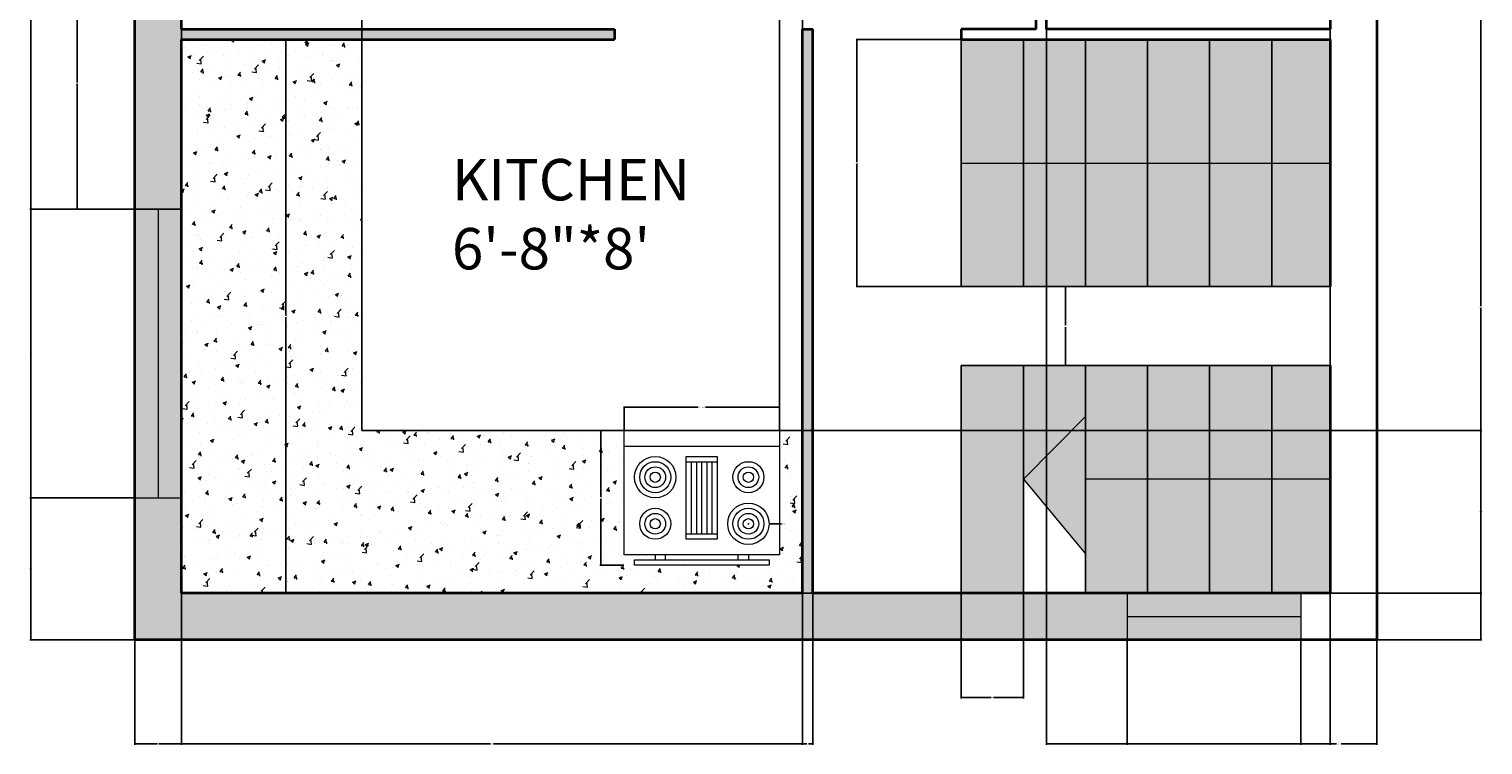
# Model space of a CAD drawing. Units: inches. Extents: x 17031430 to 17032061, y 16082759 to 16083238.
# Tile 1 of 3: x 17031435 to 17031716, y 16082759 to 16082898. Entities that reach past the tile are written whole.
import ezdxf

# ---------------------------------------------------------------- set-up
doc = ezdxf.new("R2010")
doc.units = ezdxf.units.IN
doc.header["$MEASUREMENT"] = 0
for name, color, linetype, lineweight in [('A-ANNO-DIMS', 2, 'Continuous', 18), ('A-AREA-IDEN', 7, 'Continuous', 25), ('A-EQPM', 8, 'Continuous', 18), ('A-FLOR-CASE', 8, 'Continuous', 25), ('A-FLOR-STRS', 7, 'Continuous', 25), ('A-FLOR-STRS-PATT', 254, 'Continuous', 13), ('A-GLAZ', 4, 'Continuous', 18), ('A-WALL', 7, 'Continuous', 35)]:
    doc.layers.add(name, color=color, linetype=linetype, lineweight=lineweight)
for name, color, linetype, lineweight, true_color in [('A-ANNO-SYMB', 116, 'Continuous', 18, 0x136734), ('A-ANNO-SYMB-PATT', 116, 'Continuous', 13, 0x136734), ('A-FLOR-CASE-PATT', 9, 'Continuous', 13, 0xc7c8ca), ('A-GLAZ-PATT', 252, 'Continuous', 13, 0x939598), ('A-WALL-PATT', 18, 'Continuous', 13, 0x000000)]:
    doc.layers.add(name, color=color, linetype=linetype, lineweight=lineweight, true_color=true_color)
doc.styles.get("Standard").update_dxf_attribs({"font": 'arial.ttf'})
doc.dimstyles.get("Standard").update_dxf_attribs({"dimtxt": 0.18, "dimasz": 0.18, "dimexe": 0.18, "dimexo": 0.0625, "dimgap": 0.09, "dimtad": 0, "dimtih": 1, "dimtoh": 1, "dimdec": 0, "dimzin": 0, "dimdsep": 46, "dimlunit": 3, "dimtxsty": 'Standard', "dimcen": 0.09, "dimadec": 0, "dimazin": 0, "dimtfac": 1, "dimtdec": 0, "dimtofl": 0, "dimtmove": 0, "dimatfit": 3, "dimfxl": 1, "dimtolj": 1, "dimtzin": 0, "dimarcsym": 0})

# ---------------------------------------------------------------- blocks, each defined once
blk = doc.blocks.new('Range-Oven - 30 in top')
for p, q in [((0, -3), (30, -3)), ((12, -6), (18, -6)), ((13, -20), (13, -6)), ((14, -6), (14, -20)), ((15, -20), (15, -6)), ((16, -6), (16, -20)), ((17, -20), (17, -6)), ((18, -20), (12, -20)), ((6, -24), (6, -25)), ((8, -25), (8, -24)), ((22, -25), (22, -24)), ((24, -24), (24, -25))]:
    blk.add_line(p, q)
for points in [[(0, -24), (0, 0), (30, 0), (30, -24)], [(12, -21), (12, -5), (18, -5), (18, -21)], [(2, -26), (2, -25), (28, -25), (28, -26)]]:
    blk.add_lwpolyline(points, close=True)
for centre, radius in [((6, -9), 4), ((6, -9), 3), ((6, -9), 2), ((6, -9), 1), ((24, -9), 3), ((24, -9), 2), ((24, -9), 1), ((24, -18), 4), ((6, -18), 3), ((6, -18), 2), ((24, -18), 3), ((24, -18), 2), ((6, -18), 1), ((24, -18), 1)]:
    blk.add_circle(centre, radius)
blk = doc.blocks.new('*D12')
at = {"layer": 'A-ANNO-DIMS', "color": 0, "lineweight": -2, "transparency": 16777216}
for p, q in [((17031550.32, 16082820.21), (17031550.32, 16082824.83)), ((17031550.5, 16082824.65), (17031564.62, 16082824.65)), ((17031580.14, 16082824.65), (17031566.01, 16082824.65)), ((17031580.32, 16082820.21), (17031580.32, 16082824.83))]:
    blk.add_line(p, q, dxfattribs=at)
at = {"layer": 'A-ANNO-DIMS', "color": 0, "transparency": 16777216}
for points in [[(17031550.5, 16082824.68), (17031550.5, 16082824.62), (17031550.32, 16082824.65)], [(17031580.14, 16082824.68), (17031580.14, 16082824.62), (17031580.32, 16082824.65)]]:
    blk.add_solid(points, dxfattribs=at)
at = {"layer": 'Defpoints', "color": 0, "transparency": 16777216}
for p in [(17031580.32, 16082824.65), (17031550.32, 16082820.15), (17031580.32, 16082820.15)]:
    blk.add_point(p, dxfattribs=at)
at = {"layer": 'A-ANNO-DIMS', "color": 0, "transparency": 16777216, "insert": (17031565.32, 16082824.65), "char_height": 0.18, "attachment_point": 5}
blk.add_mtext('\\A1;RANGE 30', dxfattribs=at)
blk = doc.blocks.new('*D13')
at = {"layer": 'A-ANNO-DIMS', "color": 0, "lineweight": -2, "transparency": 16777216}
for p, q in [((17031550.25, 16082820.15), (17031545.64, 16082820.15)), ((17031545.82, 16082819.97), (17031545.82, 16082807.33)), ((17031545.82, 16082794.33), (17031545.82, 16082806.96)), ((17031550.25, 16082794.15), (17031545.64, 16082794.15))]:
    blk.add_line(p, q, dxfattribs=at)
at = {"layer": 'A-ANNO-DIMS', "color": 0, "transparency": 16777216}
for points in [[(17031545.79, 16082819.97), (17031545.85, 16082819.97), (17031545.82, 16082820.15)], [(17031545.79, 16082794.33), (17031545.85, 16082794.33), (17031545.82, 16082794.15)]]:
    blk.add_solid(points, dxfattribs=at)
at = {"layer": 'Defpoints', "color": 0, "transparency": 16777216}
for p in [(17031545.82, 16082820.15), (17031550.32, 16082820.15), (17031550.32, 16082794.15)]:
    blk.add_point(p, dxfattribs=at)
at = {"layer": 'A-ANNO-DIMS', "color": 0, "transparency": 16777216, "insert": (17031545.82, 16082807.15), "char_height": 0.18, "attachment_point": 5}
blk.add_mtext('\\A1;26', dxfattribs=at)
blk = doc.blocks.new('*D15')
at = {"layer": 'A-ANNO-DIMS', "color": 0, "lineweight": -2, "transparency": 16777216}
for p, q in [((17031455.69, 16083139.74), (17031435.43, 16083139.74)), ((17031435.61, 16083139.56), (17031435.61, 16082959.92)), ((17031435.61, 16082779.92), (17031435.61, 16082959.56)), ((17031455.69, 16082779.74), (17031435.43, 16082779.74))]:
    blk.add_line(p, q, dxfattribs=at)
at = {"layer": 'A-ANNO-DIMS', "color": 0, "transparency": 16777216}
for points in [[(17031435.58, 16083139.56), (17031435.64, 16083139.56), (17031435.61, 16083139.74)], [(17031435.58, 16082779.92), (17031435.64, 16082779.92), (17031435.61, 16082779.74)]]:
    blk.add_solid(points, dxfattribs=at)
at = {"layer": 'Defpoints', "color": 0, "transparency": 16777216}
for p in [(17031435.61, 16083139.74), (17031455.76, 16083139.74), (17031455.76, 16082779.74)]:
    blk.add_point(p, dxfattribs=at)
at = {"layer": 'A-ANNO-DIMS', "color": 0, "transparency": 16777216, "insert": (17031435.61, 16082959.74), "char_height": 0.18, "attachment_point": 5}
blk.add_mtext('\\A1;360', dxfattribs=at)
blk = doc.blocks.new('*D19')
at = {"layer": 'A-ANNO-DIMS', "color": 0, "lineweight": -2, "transparency": 16777216}
for p, q in [((17031647.53, 16082779.68), (17031647.53, 16082759.41)), ((17031681.1, 16082779.68), (17031681.1, 16082759.41)), ((17031647.71, 16082759.59), (17031663.85, 16082759.59)), ((17031680.92, 16082759.59), (17031664.78, 16082759.59))]:
    blk.add_line(p, q, dxfattribs=at)
at = {"layer": 'A-ANNO-DIMS', "color": 0, "transparency": 16777216}
for points in [[(17031647.71, 16082759.62), (17031647.71, 16082759.56), (17031647.53, 16082759.59)], [(17031680.92, 16082759.62), (17031680.92, 16082759.56), (17031681.1, 16082759.59)]]:
    blk.add_solid(points, dxfattribs=at)
at = {"layer": 'Defpoints', "color": 0, "transparency": 16777216}
for p in [(17031647.53, 16082779.74), (17031681.1, 16082779.74), (17031681.1, 16082759.59)]:
    blk.add_point(p, dxfattribs=at)
at = {"layer": 'A-ANNO-DIMS', "color": 0, "transparency": 16777216, "insert": (17031664.31, 16082759.59), "char_height": 0.18, "attachment_point": 5}
blk.add_mtext('\\A1;33.567', dxfattribs=at)
blk = doc.blocks.new('*D20')
at = {"layer": 'A-ANNO-DIMS', "color": 0, "lineweight": -2, "transparency": 16777216}
for p, q in [((17031681.1, 16082779.68), (17031681.1, 16082759.41)), ((17031695.76, 16082779.68), (17031695.76, 16082759.41)), ((17031681.28, 16082759.59), (17031687.97, 16082759.59)), ((17031695.58, 16082759.59), (17031688.88, 16082759.59))]:
    blk.add_line(p, q, dxfattribs=at)
at = {"layer": 'A-ANNO-DIMS', "color": 0, "transparency": 16777216}
for points in [[(17031681.28, 16082759.62), (17031681.28, 16082759.56), (17031681.1, 16082759.59)], [(17031695.58, 16082759.62), (17031695.58, 16082759.56), (17031695.76, 16082759.59)]]:
    blk.add_solid(points, dxfattribs=at)
at = {"layer": 'Defpoints', "color": 0, "transparency": 16777216}
for p in [(17031681.1, 16082779.74), (17031695.76, 16082779.74), (17031695.76, 16082759.59)]:
    blk.add_point(p, dxfattribs=at)
at = {"layer": 'A-ANNO-DIMS', "color": 0, "transparency": 16777216, "insert": (17031688.43, 16082759.59), "char_height": 0.18, "attachment_point": 5}
blk.add_mtext('\\A1;14.662', dxfattribs=at)
blk = doc.blocks.new('*D21')
at = {"layer": 'A-ANNO-DIMS', "color": 0, "lineweight": -2, "transparency": 16777216}
for p, q in [((17031455.69, 16082807.18), (17031435.43, 16082807.18)), ((17031435.61, 16082807), (17031435.61, 16082793.64)), ((17031435.61, 16082779.92), (17031435.61, 16082793.28)), ((17031455.69, 16082779.74), (17031435.43, 16082779.74))]:
    blk.add_line(p, q, dxfattribs=at)
at = {"layer": 'A-ANNO-DIMS', "color": 0, "transparency": 16777216}
for points in [[(17031435.58, 16082807), (17031435.64, 16082807), (17031435.61, 16082807.18)], [(17031435.58, 16082779.92), (17031435.64, 16082779.92), (17031435.61, 16082779.74)]]:
    blk.add_solid(points, dxfattribs=at)
at = {"layer": 'Defpoints', "color": 0, "transparency": 16777216}
for p in [(17031435.61, 16082807.18), (17031455.76, 16082807.18), (17031455.76, 16082779.74)]:
    blk.add_point(p, dxfattribs=at)
at = {"layer": 'A-ANNO-DIMS', "color": 0, "transparency": 16777216, "insert": (17031435.61, 16082793.46), "char_height": 0.18, "attachment_point": 5}
blk.add_mtext('\\A1;27.44', dxfattribs=at)
blk = doc.blocks.new('*D22')
at = {"layer": 'A-ANNO-DIMS', "color": 0, "lineweight": -2, "transparency": 16777216}
for p, q in [((17031455.69, 16082862.95), (17031435.43, 16082862.95)), ((17031435.61, 16082862.77), (17031435.61, 16082835.25)), ((17031435.61, 16082807.36), (17031435.61, 16082834.89)), ((17031455.69, 16082807.18), (17031435.43, 16082807.18))]:
    blk.add_line(p, q, dxfattribs=at)
at = {"layer": 'A-ANNO-DIMS', "color": 0, "transparency": 16777216}
for points in [[(17031435.58, 16082862.77), (17031435.64, 16082862.77), (17031435.61, 16082862.95)], [(17031435.58, 16082807.36), (17031435.64, 16082807.36), (17031435.61, 16082807.18)]]:
    blk.add_solid(points, dxfattribs=at)
at = {"layer": 'Defpoints', "color": 0, "transparency": 16777216}
for p in [(17031435.61, 16082862.95), (17031455.76, 16082862.95), (17031455.76, 16082807.18)]:
    blk.add_point(p, dxfattribs=at)
at = {"layer": 'A-ANNO-DIMS', "color": 0, "transparency": 16777216, "insert": (17031435.61, 16082835.07), "char_height": 0.18, "attachment_point": 5}
blk.add_mtext('\\A1;55.77', dxfattribs=at)
blk = doc.blocks.new('*D23')
at = {"layer": 'A-ANNO-DIMS', "color": 0, "lineweight": -2, "transparency": 16777216}
for p, q in [((17031464.69, 16082911.7), (17031444.43, 16082911.7)), ((17031444.61, 16082911.52), (17031444.61, 16082887.51)), ((17031444.61, 16082863.13), (17031444.61, 16082887.14)), ((17031464.69, 16082862.95), (17031444.43, 16082862.95))]:
    blk.add_line(p, q, dxfattribs=at)
at = {"layer": 'A-ANNO-DIMS', "color": 0, "transparency": 16777216}
for points in [[(17031444.58, 16082911.52), (17031444.64, 16082911.52), (17031444.61, 16082911.7)], [(17031444.58, 16082863.13), (17031444.64, 16082863.13), (17031444.61, 16082862.95)]]:
    blk.add_solid(points, dxfattribs=at)
at = {"layer": 'Defpoints', "color": 0, "transparency": 16777216}
for p in [(17031444.61, 16082911.7), (17031464.76, 16082911.7), (17031464.76, 16082862.95)]:
    blk.add_point(p, dxfattribs=at)
at = {"layer": 'A-ANNO-DIMS', "color": 0, "transparency": 16777216, "insert": (17031444.61, 16082887.33), "char_height": 0.18, "attachment_point": 5}
blk.add_mtext('\\A1;48.74', dxfattribs=at)
blk = doc.blocks.new('*D27')
at = {"layer": 'A-ANNO-DIMS', "color": 0, "lineweight": -2, "transparency": 16777216}
for p, q in [((17031695.82, 16082908.33), (17031716.09, 16082908.33)), ((17031715.91, 16082908.15), (17031715.91, 16082844.22)), ((17031715.91, 16082779.92), (17031715.91, 16082843.85)), ((17031695.82, 16082779.74), (17031716.09, 16082779.74))]:
    blk.add_line(p, q, dxfattribs=at)
at = {"layer": 'A-ANNO-DIMS', "color": 0, "transparency": 16777216}
for points in [[(17031715.88, 16082908.15), (17031715.94, 16082908.15), (17031715.91, 16082908.33)], [(17031715.88, 16082779.92), (17031715.94, 16082779.92), (17031715.91, 16082779.74)]]:
    blk.add_solid(points, dxfattribs=at)
at = {"layer": 'Defpoints', "color": 0, "transparency": 16777216}
for p in [(17031695.76, 16082908.33), (17031695.76, 16082779.74), (17031715.91, 16082779.74)]:
    blk.add_point(p, dxfattribs=at)
at = {"layer": 'A-ANNO-DIMS', "color": 0, "transparency": 16777216, "insert": (17031715.91, 16082844.04), "char_height": 0.18, "attachment_point": 5}
blk.add_mtext('\\A1;128.6', dxfattribs=at)
blk = doc.blocks.new('*D33')
at = {"layer": 'A-ANNO-DIMS', "color": 0, "lineweight": -2, "transparency": 16777216}
for p, q in [((17031464.76, 16082788.68), (17031464.76, 16082759.41)), ((17031455.76, 16082779.68), (17031455.76, 16082759.41)), ((17031455.94, 16082759.59), (17031460.11, 16082759.59)), ((17031464.58, 16082759.59), (17031460.41, 16082759.59))]:
    blk.add_line(p, q, dxfattribs=at)
at = {"layer": 'A-ANNO-DIMS', "color": 0, "transparency": 16777216}
for points in [[(17031455.94, 16082759.62), (17031455.94, 16082759.56), (17031455.76, 16082759.59)], [(17031464.58, 16082759.62), (17031464.58, 16082759.56), (17031464.76, 16082759.59)]]:
    blk.add_solid(points, dxfattribs=at)
at = {"layer": 'Defpoints', "color": 0, "transparency": 16777216}
for p in [(17031464.76, 16082788.74), (17031455.76, 16082779.74), (17031464.76, 16082759.59)]:
    blk.add_point(p, dxfattribs=at)
at = {"layer": 'A-ANNO-DIMS', "color": 0, "transparency": 16777216, "insert": (17031460.26, 16082759.59), "char_height": 0.18, "attachment_point": 5}
blk.add_mtext('\\A1;9', dxfattribs=at)
blk = doc.blocks.new('*D34')
at = {"layer": 'A-ANNO-DIMS', "color": 0, "lineweight": -2, "transparency": 16777216}
for p, q in [((17031464.76, 16082788.68), (17031464.76, 16082759.41)), ((17031584.76, 16082788.68), (17031584.76, 16082759.41)), ((17031464.94, 16082759.59), (17031524.48, 16082759.59)), ((17031584.58, 16082759.59), (17031525.04, 16082759.59))]:
    blk.add_line(p, q, dxfattribs=at)
at = {"layer": 'A-ANNO-DIMS', "color": 0, "transparency": 16777216}
for points in [[(17031464.94, 16082759.62), (17031464.94, 16082759.56), (17031464.76, 16082759.59)], [(17031584.58, 16082759.62), (17031584.58, 16082759.56), (17031584.76, 16082759.59)]]:
    blk.add_solid(points, dxfattribs=at)
at = {"layer": 'Defpoints', "color": 0, "transparency": 16777216}
for p in [(17031464.76, 16082788.74), (17031584.76, 16082788.74), (17031584.76, 16082759.59)]:
    blk.add_point(p, dxfattribs=at)
at = {"layer": 'A-ANNO-DIMS', "color": 0, "transparency": 16777216, "insert": (17031524.76, 16082759.59), "char_height": 0.18, "attachment_point": 5}
blk.add_mtext('\\A1;120', dxfattribs=at)
blk = doc.blocks.new('*D35')
at = {"layer": 'A-ANNO-DIMS', "color": 0, "lineweight": -2, "transparency": 16777216}
for p, q in [((17031584.76, 16082788.68), (17031584.76, 16082759.41)), ((17031586.76, 16082788.68), (17031586.76, 16082759.41)), ((17031584.94, 16082759.59), (17031585.61, 16082759.59)), ((17031586.58, 16082759.59), (17031585.91, 16082759.59))]:
    blk.add_line(p, q, dxfattribs=at)
at = {"layer": 'A-ANNO-DIMS', "color": 0, "transparency": 16777216}
for points in [[(17031584.94, 16082759.62), (17031584.94, 16082759.56), (17031584.76, 16082759.59)], [(17031586.58, 16082759.62), (17031586.58, 16082759.56), (17031586.76, 16082759.59)]]:
    blk.add_solid(points, dxfattribs=at)
at = {"layer": 'Defpoints', "color": 0, "transparency": 16777216}
for p in [(17031584.76, 16082788.74), (17031586.76, 16082788.74), (17031586.76, 16082759.59)]:
    blk.add_point(p, dxfattribs=at)
at = {"layer": 'A-ANNO-DIMS', "color": 0, "transparency": 16777216, "insert": (17031585.76, 16082759.59), "char_height": 0.18, "attachment_point": 5}
blk.add_mtext('\\A1;2', dxfattribs=at)
blk = doc.blocks.new('*D36')
at = {"layer": 'A-ANNO-DIMS', "color": 0, "lineweight": -2, "transparency": 16777216}
for p, q in [((17031464.82, 16082895.74), (17031485.09, 16082895.74)), ((17031484.91, 16082895.56), (17031484.91, 16082842.42)), ((17031484.91, 16082788.92), (17031484.91, 16082842.06)), ((17031464.82, 16082788.74), (17031485.09, 16082788.74))]:
    blk.add_line(p, q, dxfattribs=at)
at = {"layer": 'A-ANNO-DIMS', "color": 0, "transparency": 16777216}
for points in [[(17031484.88, 16082895.56), (17031484.94, 16082895.56), (17031484.91, 16082895.74)], [(17031484.88, 16082788.92), (17031484.94, 16082788.92), (17031484.91, 16082788.74)]]:
    blk.add_solid(points, dxfattribs=at)
at = {"layer": 'Defpoints', "color": 0, "transparency": 16777216}
for p in [(17031464.76, 16082895.74), (17031464.76, 16082788.74), (17031484.91, 16082788.74)]:
    blk.add_point(p, dxfattribs=at)
at = {"layer": 'A-ANNO-DIMS', "color": 0, "transparency": 16777216, "insert": (17031484.91, 16082842.24), "char_height": 0.18, "attachment_point": 5}
blk.add_mtext('\\A1;107', dxfattribs=at)
blk = doc.blocks.new('*D43')
at = {"layer": 'A-ANNO-DIMS', "color": 0, "lineweight": -2, "transparency": 16777216}
for p, q in [((17031631.91, 16082897.68), (17031631.91, 16082759.41)), ((17031686.76, 16082897.68), (17031686.76, 16082759.41)), ((17031632.09, 16082759.59), (17031658.94, 16082759.59)), ((17031686.58, 16082759.59), (17031659.73, 16082759.59))]:
    blk.add_line(p, q, dxfattribs=at)
at = {"layer": 'A-ANNO-DIMS', "color": 0, "transparency": 16777216}
for points in [[(17031632.09, 16082759.62), (17031632.09, 16082759.56), (17031631.91, 16082759.59)], [(17031686.58, 16082759.62), (17031686.58, 16082759.56), (17031686.76, 16082759.59)]]:
    blk.add_solid(points, dxfattribs=at)
at = {"layer": 'Defpoints', "color": 0, "transparency": 16777216}
for p in [(17031631.91, 16082897.74), (17031686.76, 16082897.74), (17031686.76, 16082759.59)]:
    blk.add_point(p, dxfattribs=at)
at = {"layer": 'A-ANNO-DIMS', "color": 0, "transparency": 16777216, "insert": (17031659.34, 16082759.59), "char_height": 0.18, "attachment_point": 5}
blk.add_mtext('\\A1;54.84', dxfattribs=at)
blk = doc.blocks.new('*D45')
at = {"layer": 'A-ANNO-DIMS', "color": 0, "lineweight": -2, "transparency": 16777216}
for p, q in [((17031464.76, 16082895.8), (17031464.76, 16083160.07)), ((17031464.94, 16083159.89), (17031481.79, 16083159.89)), ((17031499.44, 16083159.89), (17031482.58, 16083159.89)), ((17031499.62, 16082895.8), (17031499.62, 16083160.07))]:
    blk.add_line(p, q, dxfattribs=at)
at = {"layer": 'A-ANNO-DIMS', "color": 0, "transparency": 16777216}
for points in [[(17031464.94, 16083159.92), (17031464.94, 16083159.86), (17031464.76, 16083159.89)], [(17031499.44, 16083159.92), (17031499.44, 16083159.86), (17031499.62, 16083159.89)]]:
    blk.add_solid(points, dxfattribs=at)
at = {"layer": 'Defpoints', "color": 0, "transparency": 16777216}
for p in [(17031499.62, 16083159.89), (17031464.76, 16082895.74), (17031499.62, 16082895.74)]:
    blk.add_point(p, dxfattribs=at)
at = {"layer": 'A-ANNO-DIMS', "color": 0, "transparency": 16777216, "insert": (17031482.19, 16083159.89), "char_height": 0.18, "attachment_point": 5}
blk.add_mtext('\\A1;34.86', dxfattribs=at)
blk = doc.blocks.new('*D46')
at = {"layer": 'A-ANNO-DIMS', "color": 0, "lineweight": -2, "transparency": 16777216}
for p, q in [((17031584.82, 16082820.15), (17031716.09, 16082820.15)), ((17031715.91, 16082819.97), (17031715.91, 16082804.63)), ((17031715.91, 16082788.92), (17031715.91, 16082804.26)), ((17031584.82, 16082788.74), (17031716.09, 16082788.74))]:
    blk.add_line(p, q, dxfattribs=at)
at = {"layer": 'A-ANNO-DIMS', "color": 0, "transparency": 16777216}
for points in [[(17031715.88, 16082819.97), (17031715.94, 16082819.97), (17031715.91, 16082820.15)], [(17031715.88, 16082788.92), (17031715.94, 16082788.92), (17031715.91, 16082788.74)]]:
    blk.add_solid(points, dxfattribs=at)
at = {"layer": 'Defpoints', "color": 0, "transparency": 16777216}
for p in [(17031584.76, 16082820.15), (17031584.76, 16082788.74), (17031715.91, 16082788.74)]:
    blk.add_point(p, dxfattribs=at)
at = {"layer": 'A-ANNO-DIMS', "color": 0, "transparency": 16777216, "insert": (17031715.91, 16082804.44), "char_height": 0.18, "attachment_point": 5}
blk.add_mtext('\\A1;31.405', dxfattribs=at)
blk = doc.blocks.new('*D47')
at = {"layer": 'A-ANNO-DIMS', "color": 0, "lineweight": -2, "transparency": 16777216}
for p, q in [((17031580.32, 16082820.21), (17031580.32, 16083160.07)), ((17031580.5, 16083159.89), (17031582.16, 16083159.89)), ((17031584.58, 16083159.89), (17031582.92, 16083159.89)), ((17031584.76, 16082820.21), (17031584.76, 16083160.07))]:
    blk.add_line(p, q, dxfattribs=at)
at = {"layer": 'A-ANNO-DIMS', "color": 0, "transparency": 16777216}
for points in [[(17031580.5, 16083159.92), (17031580.5, 16083159.86), (17031580.32, 16083159.89)], [(17031584.58, 16083159.92), (17031584.58, 16083159.86), (17031584.76, 16083159.89)]]:
    blk.add_solid(points, dxfattribs=at)
at = {"layer": 'Defpoints', "color": 0, "transparency": 16777216}
for p in [(17031584.76, 16083159.89), (17031580.32, 16082820.15), (17031584.76, 16082820.15)]:
    blk.add_point(p, dxfattribs=at)
at = {"layer": 'A-ANNO-DIMS', "color": 0, "transparency": 16777216, "insert": (17031582.54, 16083159.89), "char_height": 0.18, "attachment_point": 5}
blk.add_mtext('\\A1;4.441', dxfattribs=at)
blk = doc.blocks.new('*D48')
at = {"layer": 'A-ANNO-DIMS', "color": 0, "lineweight": -2, "transparency": 16777216}
for p, q in [((17031615.4, 16082895.74), (17031595.13, 16082895.74)), ((17031595.31, 16082895.56), (17031595.31, 16082872.03)), ((17031595.31, 16082848.15), (17031595.31, 16082871.67)), ((17031615.4, 16082847.97), (17031595.13, 16082847.97))]:
    blk.add_line(p, q, dxfattribs=at)
at = {"layer": 'A-ANNO-DIMS', "color": 0, "transparency": 16777216}
for points in [[(17031595.28, 16082895.56), (17031595.34, 16082895.56), (17031595.31, 16082895.74)], [(17031595.28, 16082848.15), (17031595.34, 16082848.15), (17031595.31, 16082847.97)]]:
    blk.add_solid(points, dxfattribs=at)
at = {"layer": 'Defpoints', "color": 0, "transparency": 16777216}
for p in [(17031595.31, 16082895.74), (17031615.46, 16082895.74), (17031615.46, 16082847.97)]:
    blk.add_point(p, dxfattribs=at)
at = {"layer": 'A-ANNO-DIMS', "color": 0, "transparency": 16777216, "insert": (17031595.31, 16082871.85), "char_height": 0.18, "attachment_point": 5}
blk.add_mtext('\\A1;47.77', dxfattribs=at)
blk = doc.blocks.new('*D49')
at = {"layer": 'A-ANNO-DIMS', "color": 0, "lineweight": -2, "transparency": 16777216}
for p, q in [((17031615.53, 16082847.97), (17031635.79, 16082847.97)), ((17031635.61, 16082847.79), (17031635.61, 16082840.54)), ((17031635.61, 16082832.92), (17031635.61, 16082840.17)), ((17031615.53, 16082832.74), (17031635.79, 16082832.74))]:
    blk.add_line(p, q, dxfattribs=at)
at = {"layer": 'A-ANNO-DIMS', "color": 0, "transparency": 16777216}
for points in [[(17031635.58, 16082847.79), (17031635.64, 16082847.79), (17031635.61, 16082847.97)], [(17031635.58, 16082832.92), (17031635.64, 16082832.92), (17031635.61, 16082832.74)]]:
    blk.add_solid(points, dxfattribs=at)
at = {"layer": 'Defpoints', "color": 0, "transparency": 16777216}
for p in [(17031615.46, 16082847.97), (17031615.46, 16082832.74), (17031635.61, 16082832.74)]:
    blk.add_point(p, dxfattribs=at)
at = {"layer": 'A-ANNO-DIMS', "color": 0, "transparency": 16777216, "insert": (17031635.61, 16082840.36), "char_height": 0.18, "attachment_point": 5}
blk.add_mtext('\\A1;15.226', dxfattribs=at)
blk = doc.blocks.new('*D50')
at = {"layer": 'A-ANNO-DIMS', "color": 0, "lineweight": -2, "transparency": 16777216}
for p, q in [((17031615.46, 16082788.68), (17031615.46, 16082768.41)), ((17031627.46, 16082788.68), (17031627.46, 16082768.41)), ((17031615.64, 16082768.59), (17031621.26, 16082768.59)), ((17031627.28, 16082768.59), (17031621.67, 16082768.59))]:
    blk.add_line(p, q, dxfattribs=at)
at = {"layer": 'A-ANNO-DIMS', "color": 0, "transparency": 16777216}
for points in [[(17031615.64, 16082768.62), (17031615.64, 16082768.56), (17031615.46, 16082768.59)], [(17031627.28, 16082768.62), (17031627.28, 16082768.56), (17031627.46, 16082768.59)]]:
    blk.add_solid(points, dxfattribs=at)
at = {"layer": 'Defpoints', "color": 0, "transparency": 16777216}
for p in [(17031615.46, 16082788.74), (17031627.46, 16082788.74), (17031615.46, 16082768.59)]:
    blk.add_point(p, dxfattribs=at)
at = {"layer": 'A-ANNO-DIMS', "color": 0, "transparency": 16777216, "insert": (17031621.46, 16082768.59), "char_height": 0.18, "attachment_point": 5}
blk.add_mtext('\\A1;12', dxfattribs=at)
blk = doc.blocks.new('*D61')
at = {"layer": 'A-ANNO-DIMS', "color": 0, "lineweight": -2, "transparency": 16777216}
for p, q in [((17031574.23, 16082802.15), (17031574.41, 16082802.15)), ((17031574.32, 16082802.06), (17031574.32, 16082802.24)), ((17031580.72, 16082802.15), (17031578.5, 16082802.15))]:
    blk.add_line(p, q, dxfattribs=at)
at = {"layer": 'A-ANNO-DIMS', "color": 0, "transparency": 16777216}
blk.add_solid([(17031578.5, 16082802.18), (17031578.5, 16082802.12), (17031578.32, 16082802.15)], dxfattribs=at)
at = {"layer": 'Defpoints', "color": 0, "transparency": 16777216}
for p in [(17031570.32, 16082802.15), (17031578.32, 16082802.15)]:
    blk.add_point(p, dxfattribs=at)
at = {"layer": 'A-ANNO-DIMS', "color": 0, "transparency": 16777216, "insert": (17031581.15, 16082802.15), "char_height": 0.18, "attachment_point": 5}
blk.add_mtext('\\A1;2X ∅8', dxfattribs=at)

msp = doc.modelspace()

# ---------------------------------------------------------------- hatches: boundary and pattern name
at = {"layer": 'A-ANNO-SYMB-PATT'}
h = msp.add_hatch(color=256, dxfattribs=at)
h.dxf.hatch_style = 1
h.paths.add_polyline_path([(17031639.4649, 16082822.8981), (17031627.4649, 16082810.7418), (17031639.4649, 16082796.3281)])
at = {"layer": 'A-FLOR-CASE-PATT'}
h = msp.add_hatch(dxfattribs=at)
h.set_pattern_fill('AR-CONC', color=256)
h.set_pattern_definition([(50, (0, 0), (7.172601826, -0.6275213498), [0.75, -8.25]), (355, (0, 0), (-1.3875133361, 7.521921337), [0.6, -6.6]), (100.45144446, (0.598, -0.052), (5.7850884673, 6.8943999097), [0.63740192, -7.01142112]), (46.1842, (0, 2), (10.6724133067, -1.655192808), [1.125, -12.375]), (96.63563549, (0.889, 1.862), (9.3466194567, 9.7411860077), [0.95610342, -10.5171376]), (351.18416399, (0, 2), (9.3466194505, 9.7411860027), [0.9, -9.90000001]), (21, (1, 1.5), (5.9690705212, -4.0261889067), [0.75, -8.25]), (326, (1, 1.5), (2.4331533192, 7.2515004505), [0.6, -6.6]), (71.45144474, (1.4974, 1.1645), (8.4022237673, 3.225311528), [0.6374019, -7.01142112]), (37.5, (0, 0), (0.12159855317, 3.3289385383), [0, -6.52, 0, -6.7, 0, -6.625]), (7.5, (0, 0), (2.6306953744, 3.9441171188), [0, -3.82, 0, -6.37, 0, -2.525]), (327.5, (-2.23, 0), (5.33822436172, -0.22554871734), [0, -2.5, 0, -7.8, 0, -10.35]), (317.5, (-3.23, 0), (5.8318616934, 1.0010498233), [0, -3.25, 0, -5.18, 0, -7.35])])
h.paths.add_polyline_path([(17031499.6182, 16082895.7405), (17031464.7571, 16082895.7405), (17031464.7571, 16082788.7405), (17031584.7571, 16082788.7405), (17031584.7571, 16082820.1456), (17031580.3158, 16082820.1456), (17031580.3158, 16082796.1456), (17031574.3158, 16082796.1456), (17031574.3158, 16082795.1456), (17031578.3158, 16082795.1456), (17031578.3158, 16082794.1456), (17031552.3158, 16082794.1456), (17031552.3158, 16082795.1456), (17031556.3158, 16082795.1456), (17031556.3158, 16082796.1456), (17031550.3158, 16082796.1456), (17031550.3158, 16082820.1456), (17031499.6182, 16082820.1456)])
at = {"layer": 'A-FLOR-STRS-PATT'}
h = msp.add_hatch(color=256, dxfattribs=at)
h.set_gradient(color1=(0, 0, 255), color2=(255, 255, 0))
h.paths.add_polyline_path([(17031627.4649, 16082895.7405), (17031615.4649, 16082895.7405), (17031615.4649, 16082871.8549), (17031627.4649, 16082871.8549)])
h.paths.add_polyline_path([(17031639.4649, 16082895.7405), (17031627.4649, 16082895.7405), (17031627.4649, 16082871.8549), (17031639.4649, 16082871.8549)])
h.paths.add_polyline_path([(17031651.4649, 16082895.7405), (17031639.4649, 16082895.7405), (17031639.4649, 16082871.8549), (17031651.4649, 16082871.8549)])
h.paths.add_polyline_path([(17031663.4649, 16082895.7405), (17031651.4649, 16082895.7405), (17031651.4649, 16082871.8549), (17031663.4649, 16082871.8549)])
h.paths.add_polyline_path([(17031686.7571, 16082895.7405), (17031675.4649, 16082895.7405), (17031675.4649, 16082871.8549), (17031686.7571, 16082871.8549)])
h.paths.add_polyline_path([(17031675.4649, 16082895.7405), (17031663.4649, 16082895.7405), (17031663.4649, 16082871.8549), (17031675.4649, 16082871.8549)])
h.paths.add_polyline_path([(17031686.7571, 16082871.8549), (17031675.4649, 16082871.8549), (17031675.4649, 16082847.9692), (17031686.7571, 16082847.9692)])
h.paths.add_polyline_path([(17031675.4649, 16082871.8549), (17031663.4649, 16082871.8549), (17031663.4649, 16082847.9692), (17031675.4649, 16082847.9692)])
h.paths.add_polyline_path([(17031663.4649, 16082871.8549), (17031651.4649, 16082871.8549), (17031651.4649, 16082847.9692), (17031663.4649, 16082847.9692)])
h.paths.add_polyline_path([(17031651.4649, 16082871.8549), (17031639.4649, 16082871.8549), (17031639.4649, 16082847.9692), (17031651.4649, 16082847.9692)])
h.paths.add_polyline_path([(17031639.4649, 16082871.8549), (17031627.4649, 16082871.8549), (17031627.4649, 16082847.9692), (17031639.4649, 16082847.9692)])
h.paths.add_polyline_path([(17031627.4649, 16082871.8549), (17031615.4649, 16082871.8549), (17031615.4649, 16082847.9692), (17031627.4649, 16082847.9692)])
h.paths.add_polyline_path([(17031627.4649, 16082832.743), (17031615.4649, 16082832.743), (17031615.4649, 16082788.7405), (17031627.4649, 16082788.7405)])
h.paths.add_polyline_path([(17031639.4649, 16082832.743), (17031627.4649, 16082832.743), (17031627.4649, 16082810.7418), (17031639.4649, 16082822.8981)])
h.paths.add_polyline_path([(17031651.4649, 16082832.743), (17031639.4649, 16082832.743), (17031639.4649, 16082822.8981), (17031639.4649, 16082810.7418), (17031651.4649, 16082810.7418)])
h.paths.add_polyline_path([(17031651.4649, 16082810.7418), (17031639.4649, 16082810.7418), (17031639.4649, 16082788.7405), (17031651.4649, 16082788.7405)])
h.paths.add_polyline_path([(17031663.4649, 16082832.743), (17031651.4649, 16082832.743), (17031651.4649, 16082810.7418), (17031663.4649, 16082810.7418)])
h.paths.add_polyline_path([(17031675.4649, 16082810.7418), (17031663.4649, 16082810.7418), (17031663.4649, 16082788.7405), (17031675.4649, 16082788.7405)])
h.paths.add_polyline_path([(17031675.4649, 16082832.743), (17031663.4649, 16082832.743), (17031663.4649, 16082810.7418), (17031675.4649, 16082810.7418)])
h.paths.add_polyline_path([(17031686.7571, 16082832.743), (17031675.4649, 16082832.743), (17031675.4649, 16082810.7418), (17031686.7571, 16082810.7418)])
h.paths.add_polyline_path([(17031686.7571, 16082810.7418), (17031675.4649, 16082810.7418), (17031675.4649, 16082788.7405), (17031686.7571, 16082788.7405)])
h.paths.add_polyline_path([(17031663.4649, 16082810.7418), (17031651.4649, 16082810.7418), (17031651.4649, 16082788.7405), (17031663.4649, 16082788.7405)])
at = {"layer": 'A-GLAZ-PATT'}
h = msp.add_hatch(color=256, dxfattribs=at)
h.dxf.hatch_style = 1
h.paths.add_polyline_path([(17031546.2248, 16083139.7405), (17031495.2896, 16083139.7405), (17031495.2896, 16083135.2405), (17031546.2248, 16083135.2405)])
h.paths.add_polyline_path([(17031546.2248, 16083135.2405), (17031495.2896, 16083135.2405), (17031495.2896, 16083130.7405), (17031546.2248, 16083130.7405)])
h.paths.add_polyline_path([(17031464.7571, 16083099.8263), (17031460.2571, 16083099.8263), (17031460.2571, 16083058.1685), (17031464.7571, 16083058.1685)])
h.paths.add_polyline_path([(17031460.2571, 16083099.8263), (17031455.7571, 16083099.8263), (17031455.7571, 16083058.1685), (17031460.2571, 16083058.1685)])
h.paths.add_polyline_path([(17031464.7571, 16082953.9805), (17031460.2571, 16082953.9805), (17031460.2571, 16082911.6971), (17031464.7571, 16082911.6971)])
h.paths.add_polyline_path([(17031460.2571, 16082953.9805), (17031455.7571, 16082953.9805), (17031455.7571, 16082911.6971), (17031460.2571, 16082911.6971)])
h.paths.add_polyline_path([(17031460.2571, 16082862.954), (17031455.7571, 16082862.954), (17031455.7571, 16082807.1802), (17031460.2571, 16082807.1802)])
h.paths.add_polyline_path([(17031464.7571, 16082862.954), (17031460.2571, 16082862.954), (17031460.2571, 16082807.1802), (17031464.7571, 16082807.1802)])
h.paths.add_polyline_path([(17031681.0952, 16082784.2405), (17031647.5287, 16082784.2405), (17031647.5287, 16082779.7405), (17031681.0952, 16082779.7405)])
h.paths.add_polyline_path([(17031681.0952, 16082788.7405), (17031647.5287, 16082788.7405), (17031647.5287, 16082784.2405), (17031681.0952, 16082784.2405)])
h.paths.add_polyline_path([(17031691.2571, 16083057.4652), (17031686.7571, 16083057.4652), (17031686.7571, 16083009.0162), (17031691.2571, 16083009.0162)])
h.paths.add_polyline_path([(17031514.2108, 16082846.7675), (17031567.264, 16082846.7675), (17031567.264, 16082876.6193), (17031514.2108, 16082876.6193)], flags=9)
h.paths.add_polyline_path([(17031636.4861, 16082934.711), (17031688.115, 16082934.711), (17031688.115, 16082964.5628), (17031636.4861, 16082964.5628)], flags=9)
h.paths.add_polyline_path([(17031509.9735, 16082952.8397), (17031561.3568, 16082952.8397), (17031561.3568, 16082996.1612), (17031509.9735, 16082996.1612)], flags=9)
h.paths.add_polyline_path([(17031605.4082, 16082988.2134), (17031667.1545, 16082988.2134), (17031667.1545, 16083004.6991), (17031605.4082, 16083004.6991)], flags=9)
h.paths.add_polyline_path([(17031598.2513, 16083096.6971), (17031641.5746, 16083096.6971), (17031641.5746, 16083126.5489), (17031598.2513, 16083126.5489)], flags=9)
h.paths.add_polyline_path([(17031536.0858, 16083028.4916), (17031577.5319, 16083028.4916), (17031577.5319, 16083058.3434), (17031536.0858, 16083058.3434)], flags=9)
at = {"layer": 'A-WALL-PATT'}
h = msp.add_hatch(color=256, dxfattribs=at)
h.dxf.hatch_style = 1
h.paths.add_polyline_path([(17031695.7571, 16083009.0162), (17031686.7571, 16083009.0162), (17031686.7571, 16082966.7405), (17031630.1205, 16082966.7405), (17031630.1205, 16082964.7405), (17031686.7571, 16082964.7405), (17031686.7571, 16082936.7854), (17031695.7571, 16082936.7854)])
h.paths.add_polyline_path([(17031695.7571, 16083092.6946), (17031686.7571, 16083092.6946), (17031686.7571, 16083082.7405), (17031584.7571, 16083082.7405), (17031584.7571, 16083019.7405), (17031584.7571, 16083017.7405), (17031584.7571, 16082966.7405), (17031584.7571, 16082964.7405), (17031586.7571, 16082964.7405), (17031586.7571, 16082966.7405), (17031586.7571, 16083080.7405), (17031686.7571, 16083080.7405), (17031686.7571, 16083057.4652), (17031695.7571, 16083057.4652)])
h.paths.add_polyline_path([(17031695.7571, 16083139.7405), (17031546.2248, 16083139.7405), (17031546.2248, 16083130.7405), (17031584.7571, 16083130.7405), (17031584.7571, 16083113.9162), (17031586.7571, 16083113.9162), (17031586.7571, 16083130.7405), (17031686.7571, 16083130.7405), (17031686.7571, 16083124.4975), (17031695.7571, 16083124.4975)])
h.paths.add_polyline_path([(17031495.2896, 16083139.7405), (17031455.7571, 16083139.7405), (17031455.7571, 16083099.8263), (17031464.7571, 16083099.8263), (17031464.7571, 16083130.7405), (17031495.2896, 16083130.7405)])
h.paths.add_polyline_path([(17031537.499, 16083019.7405), (17031464.7571, 16083019.7405), (17031464.7571, 16083058.1685), (17031455.7571, 16083058.1685), (17031455.7571, 16082953.9805), (17031464.7571, 16082953.9805), (17031464.7571, 16083017.7405), (17031537.499, 16083017.7405)])
h.paths.add_polyline_path([(17031464.7571, 16082911.6971), (17031455.7571, 16082911.6971), (17031455.7571, 16082862.954), (17031464.7571, 16082862.954), (17031464.7571, 16082895.7405), (17031548.467, 16082895.7405), (17031548.467, 16082897.7405), (17031464.7571, 16082897.7405)])
h.paths.add_polyline_path([(17031464.7571, 16082807.1802), (17031455.7571, 16082807.1802), (17031455.7571, 16082779.7405), (17031647.5287, 16082779.7405), (17031647.5287, 16082788.7405), (17031586.7571, 16082788.7405), (17031586.7571, 16082897.7405), (17031584.7571, 16082897.7405), (17031584.7571, 16082895.7405), (17031584.7571, 16082788.7405), (17031464.7571, 16082788.7405)])
h.paths.add_polyline_path([(17031514.2108, 16082846.7675), (17031567.264, 16082846.7675), (17031567.264, 16082876.6193), (17031514.2108, 16082876.6193)], flags=25)
h.paths.add_polyline_path([(17031636.4861, 16082934.711), (17031688.115, 16082934.711), (17031688.115, 16082964.5628), (17031636.4861, 16082964.5628)], flags=9)
h.paths.add_polyline_path([(17031509.9735, 16082952.8397), (17031561.3568, 16082952.8397), (17031561.3568, 16082996.1612), (17031509.9735, 16082996.1612)], flags=9)
h.paths.add_polyline_path([(17031605.4082, 16082988.2134), (17031667.1545, 16082988.2134), (17031667.1545, 16083004.6991), (17031605.4082, 16083004.6991)], flags=25)
h.paths.add_polyline_path([(17031598.2513, 16083096.6971), (17031641.5746, 16083096.6971), (17031641.5746, 16083126.5489), (17031598.2513, 16083126.5489)], flags=9)
h.paths.add_polyline_path([(17031536.0858, 16083028.4916), (17031577.5319, 16083028.4916), (17031577.5319, 16083058.3434), (17031536.0858, 16083058.3434)], flags=9)

# ---------------------------------------------------------------- linework, layer by layer
at = {"layer": 'A-ANNO-SYMB'}
for p, q in [((17031615.4649, 16082871.8549), (17031686.7571, 16082871.8549)), ((17031686.7571, 16082871.8549), (17031686.7571, 16082810.7418)), ((17031627.4649, 16082810.7418), (17031639.4649, 16082822.8981)), ((17031627.4649, 16082810.7418), (17031639.4649, 16082796.3281)), ((17031686.7571, 16082810.7418), (17031639.4649, 16082810.7418))]:
    msp.add_line(p, q, dxfattribs=at)
at = {"layer": 'A-FLOR-CASE'}
for p, q in [((17031499.6182, 16082895.7405), (17031499.6182, 16082820.1456)), ((17031499.6182, 16082820.1456), (17031584.7571, 16082820.1456))]:
    msp.add_line(p, q, dxfattribs=at)
at = {"layer": 'A-FLOR-STRS'}
for p, q in [((17031615.4649, 16082895.7405), (17031615.4649, 16082847.9692)), ((17031627.4649, 16082895.7405), (17031627.4649, 16082847.9692)), ((17031639.4649, 16082895.7405), (17031639.4649, 16082847.9692)), ((17031651.4649, 16082895.7405), (17031651.4649, 16082847.9692)), ((17031663.4649, 16082895.7405), (17031663.4649, 16082847.9692)), ((17031675.4649, 16082895.7405), (17031675.4649, 16082847.9692)), ((17031615.4649, 16082847.9692), (17031686.7571, 16082847.9692)), ((17031615.4649, 16082832.743), (17031686.7571, 16082832.743)), ((17031615.4649, 16082832.743), (17031615.4649, 16082788.7405)), ((17031627.4649, 16082832.743), (17031627.4649, 16082788.7405)), ((17031639.4649, 16082832.743), (17031639.4649, 16082788.7405)), ((17031651.4649, 16082832.743), (17031651.4649, 16082788.7405)), ((17031663.4649, 16082832.743), (17031663.4649, 16082788.7405)), ((17031675.4649, 16082832.743), (17031675.4649, 16082788.7405))]:
    msp.add_line(p, q, dxfattribs=at)
at = {"layer": 'A-GLAZ'}
for p, q in [((17031455.7571, 16082862.954), (17031464.7571, 16082862.954)), ((17031460.2571, 16082862.954), (17031460.2571, 16082807.1802)), ((17031455.7571, 16082807.1802), (17031464.7571, 16082807.1802)), ((17031647.5287, 16082788.7405), (17031647.5287, 16082779.7405)), ((17031681.0952, 16082788.7405), (17031681.0952, 16082779.7405)), ((17031647.5287, 16082784.2405), (17031681.0952, 16082784.2405))]:
    msp.add_line(p, q, dxfattribs=at)
at = {"layer": 'A-WALL'}
for p, q in [((17031464.7571, 16082897.7405), (17031464.7571, 16083017.7405)), ((17031686.7571, 16082964.7405), (17031686.7571, 16082897.7405)), ((17031629.9142, 16082897.7405), (17031629.9142, 16082933.7902)), ((17031631.9142, 16082897.7405), (17031631.9142, 16082933.7902)), ((17031464.7571, 16082897.7405), (17031548.467, 16082897.7405)), ((17031548.467, 16082897.7405), (17031548.467, 16082895.7405)), ((17031584.7571, 16082895.7405), (17031584.7571, 16082897.7405)), ((17031584.7571, 16082897.7405), (17031586.7571, 16082897.7405)), ((17031586.7571, 16082788.7405), (17031586.7571, 16082897.7405)), ((17031629.9142, 16082897.7405), (17031615.4649, 16082897.7405)), ((17031615.4649, 16082897.7405), (17031615.4649, 16082895.7405)), ((17031686.7571, 16082897.7405), (17031631.9142, 16082897.7405)), ((17031464.7571, 16082788.7405), (17031464.7571, 16082895.7405)), ((17031464.7571, 16082895.7405), (17031548.467, 16082895.7405)), ((17031584.7571, 16082788.7405), (17031584.7571, 16082895.7405)), ((17031615.4649, 16082895.7405), (17031686.7571, 16082895.7405)), ((17031686.7571, 16082895.7405), (17031686.7571, 16082847.9692)), ((17031686.7571, 16082832.743), (17031686.7571, 16082788.7405)), ((17031584.7571, 16082788.7405), (17031464.7571, 16082788.7405)), ((17031686.7571, 16082788.7405), (17031586.7571, 16082788.7405))]:
    msp.add_line(p, q, dxfattribs=at)
msp.add_lwpolyline([(17031695.7571, 16082779.7405), (17031455.7571, 16082779.7405), (17031455.7571, 16083139.7405), (17031695.7571, 16083139.7405)], close=True, dxfattribs=at)

# ---------------------------------------------------------------- block references
at = {"layer": 'A-EQPM'}
msp.add_blockref('Range-Oven - 30 in top', (17031550.3158, 16082820.1456), dxfattribs=at)

# ---------------------------------------------------------------- texts
at = {"layer": 'A-AREA-IDEN', "insert": (17031517.0293, 16082872.6384), "char_height": 8, "attachment_point": 1}
msp.add_mtext_dynamic_manual_height_columns('KITCHEN\\P6\'-8"*8\'', width=5.214446, gutter_width=1, heights=[0], dxfattribs=at)

# ---------------------------------------------------------------- dimensions: what is measured, and where the dimension line sits
at = {"layer": 'A-ANNO-DIMS'}
for base, p1, p2, override, picture, middle in [((17031499.6182, 16083159.8905), (17031464.7571, 16082895.7405), (17031499.6182, 16082895.7405), {"dimdec": 2, "dimlfac": 1, "dimrnd": 0, "dimzin": 0, "dimdsep": 46, "dimlunit": 2}, '*D45', (17031482.1876, 16083159.8905)), ((17031584.7571, 16083159.8905), (17031580.3158, 16082820.1456), (17031584.7571, 16082820.1456), {"dimdec": 3, "dimlfac": 1, "dimrnd": 0, "dimzin": 0, "dimdsep": 46, "dimlunit": 2}, '*D47', (17031582.5365, 16083159.8905)), ((17031686.7571, 16082759.5905), (17031631.9142, 16082897.7405), (17031686.7571, 16082897.7405), {"dimdec": 2, "dimlfac": 1, "dimrnd": 0, "dimzin": 0, "dimdsep": 46, "dimlunit": 2}, '*D43', (17031659.3357, 16082759.5905)), ((17031464.7571, 16082759.5905), (17031455.7571, 16082779.7405), (17031464.7571, 16082788.7405), {"dimdec": 0, "dimlfac": 1, "dimrnd": 0, "dimzin": 0, "dimdsep": 46, "dimlunit": 2}, '*D33', (17031460.2571, 16082759.5905)), ((17031584.7571, 16082759.5905), (17031464.7571, 16082788.7405), (17031584.7571, 16082788.7405), {"dimdec": 0, "dimlfac": 1, "dimrnd": 0, "dimzin": 0, "dimdsep": 46, "dimlunit": 2}, '*D34', (17031524.7571, 16082759.5905)), ((17031586.7571, 16082759.5905), (17031584.7571, 16082788.7405), (17031586.7571, 16082788.7405), {"dimdec": 0, "dimlfac": 1, "dimrnd": 0, "dimzin": 0, "dimdsep": 46, "dimlunit": 2}, '*D35', (17031585.7571, 16082759.5905)), ((17031681.09524, 16082759.59049), (17031647.52869, 16082779.74049), (17031681.09524, 16082779.74049), {"dimdec": 3, "dimlfac": 1, "dimrnd": 0, "dimzin": 0, "dimdsep": 46, "dimlunit": 2}, '*D19', (17031664.31196, 16082759.59049)), ((17031695.7571, 16082759.5905), (17031681.0952, 16082779.7405), (17031695.7571, 16082779.7405), {"dimdec": 3, "dimlfac": 1, "dimrnd": 0, "dimzin": 0, "dimdsep": 46, "dimlunit": 2}, '*D20', (17031688.4262, 16082759.5905))]:
    dim = msp.add_linear_dim(base=base, p1=p1, p2=p2, dimstyle='Standard', override=override, dxfattribs=at)
    dim.commit()
    dim.dimension.update_dxf_attribs({"geometry": picture, "text_midpoint": middle})
for base, p1, p2, angle, override, picture, middle in [((17031435.6071, 16083139.7405), (17031455.7571, 16082779.7405), (17031455.7571, 16083139.7405), 90, {"dimdec": 0, "dimlfac": 1, "dimrnd": 0, "dimzin": 0, "dimdsep": 46, "dimlunit": 2}, '*D15', (17031435.6071, 16082959.7405)), ((17031444.6071, 16082911.6971), (17031464.7571, 16082862.954), (17031464.7571, 16082911.6971), 90, {"dimdec": 2, "dimlfac": 1, "dimrnd": 0, "dimzin": 0, "dimdsep": 46, "dimlunit": 2}, '*D23', (17031444.6071, 16082887.3255)), ((17031715.9071, 16082779.7405), (17031695.7571, 16082908.3306), (17031695.7571, 16082779.7405), 270, {"dimdec": 1, "dimlfac": 1, "dimrnd": 0, "dimzin": 0, "dimdsep": 46, "dimlunit": 2}, '*D27', (17031715.9071, 16082844.0355)), ((17031484.9071, 16082788.7405), (17031464.7571, 16082895.7405), (17031464.7571, 16082788.7405), 270, {"dimdec": 0, "dimlfac": 1, "dimrnd": 0, "dimzin": 0, "dimdsep": 46, "dimlunit": 2}, '*D36', (17031484.9071, 16082842.2405)), ((17031595.3149, 16082895.7405), (17031615.4649, 16082847.9692), (17031615.4649, 16082895.7405), 90, {"dimdec": 2, "dimlfac": 1, "dimrnd": 0, "dimzin": 0, "dimdsep": 46, "dimlunit": 2}, '*D48', (17031595.3149, 16082871.8549)), ((17031435.6071, 16082862.954), (17031455.7571, 16082807.1802), (17031455.7571, 16082862.954), 90, {"dimdec": 2, "dimlfac": 1, "dimrnd": 0, "dimzin": 0, "dimdsep": 46, "dimlunit": 2}, '*D22', (17031435.6071, 16082835.0671)), ((17031635.6149, 16082832.743), (17031615.4649, 16082847.9692), (17031615.4649, 16082832.743), 270, {"dimdec": 3, "dimlfac": 1, "dimrnd": 0, "dimzin": 0, "dimdsep": 46, "dimlunit": 2}, '*D49', (17031635.6149, 16082840.3561)), ((17031545.8158, 16082820.1456), (17031550.3158, 16082794.1456), (17031550.3158, 16082820.1456), 90, {"dimdec": 0, "dimlfac": 1, "dimrnd": 0, "dimzin": 0, "dimdsep": 46, "dimlunit": 2}, '*D13', (17031545.8158, 16082807.1456)), ((17031715.9071, 16082788.7405), (17031584.7571, 16082820.1456), (17031584.7571, 16082788.7405), 90, {"dimdec": 3, "dimlfac": 1, "dimrnd": 0, "dimzin": 0, "dimdsep": 46, "dimlunit": 2}, '*D46', (17031715.9071, 16082804.443)), ((17031435.6071, 16082807.1802), (17031455.7571, 16082779.7405), (17031455.7571, 16082807.1802), 90, {"dimdec": 2, "dimlfac": 1, "dimrnd": 0, "dimzin": 0, "dimdsep": 46, "dimlunit": 2}, '*D21', (17031435.6071, 16082793.4603)), ((17031615.4649, 16082768.5905), (17031627.4649, 16082788.7405), (17031615.4649, 16082788.7405), 180, {"dimdec": 0, "dimlfac": 1, "dimrnd": 0, "dimzin": 0, "dimdsep": 46, "dimlunit": 2}, '*D50', (17031621.4649, 16082768.5905))]:
    dim = msp.add_linear_dim(base=base, p1=p1, p2=p2, angle=angle, dimstyle='Standard', override=override, dxfattribs=at)
    dim.commit()
    dim.dimension.update_dxf_attribs({"geometry": picture, "text_midpoint": middle})
dim = msp.add_linear_dim(base=(17031580.3158, 16082824.6456), p1=(17031550.3158, 16082820.1456), p2=(17031580.3158, 16082820.1456), text='RANGE <>', dimstyle='Standard', override={"dimdec": 0, "dimlfac": 1, "dimrnd": 0, "dimzin": 0, "dimdsep": 46, "dimlunit": 2}, dxfattribs=at)
dim.commit()
dim.dimension.update_dxf_attribs({"geometry": '*D12', "text_midpoint": (17031565.3158, 16082824.6456)})
dim = msp.add_diameter_dim_2p(p1=(17031570.3158, 16082802.1452), p2=(17031578.3158, 16082802.146), text='2X <>', dimstyle='Standard', override={"dimdec": 0, "dimlfac": 1, "dimrnd": 0, "dimzin": 0, "dimdsep": 46, "dimlunit": 2}, dxfattribs=at)
dim.commit()
dim.dimension.update_dxf_attribs({"geometry": '*D61', "text_midpoint": (17031580.7158, 16082802.1462), "dimtype": 163})

doc.saveas('drawing.dxf')
